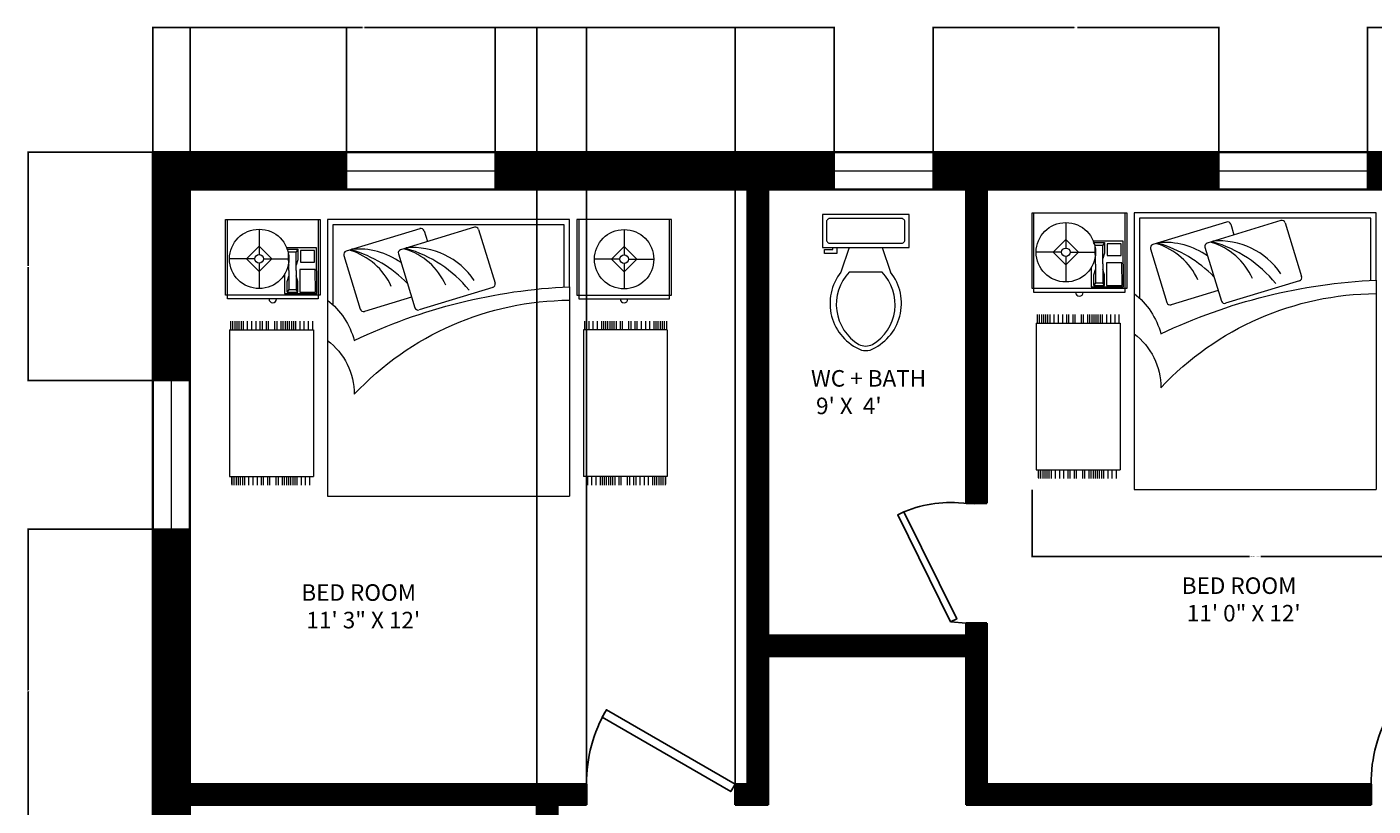
# Model space of a CAD drawing. Units: inches. Extents: x -24 to 516, y -23 to 640.
# Tile 4 of 5: x -24 to 302, y 452 to 640. Entities that reach past the tile are written whole.
import ezdxf

# ---------------------------------------------------------------- set-up
doc = ezdxf.new("R2010")
doc.units = ezdxf.units.IN
doc.header["$MEASUREMENT"] = 0
for name, color, linetype, lineweight in [('A-ANNO-DIMS', 2, 'Continuous', 18), ('A-AREA-IDEN', 7, 'Continuous', 18), ('A-WALL', 7, 'Continuous', 35), ('bathroom', 90, 'Continuous', 18), ('bedroom', 120, 'Continuous', 18), ('doors', 40, 'Continuous', 25), ('window', 30, 'Continuous', 18)]:
    doc.layers.add(name, color=color, linetype=linetype, lineweight=lineweight)
doc.layers.add('A-WALL-PATT', color=198, linetype='Continuous', lineweight=13, true_color=0x2e0f2e)
doc.styles.get("Standard").update_dxf_attribs({"font": 'arial.ttf'})
doc.dimstyles.get("Standard").update_dxf_attribs({"dimtxt": 0.18, "dimasz": 0.18, "dimexe": 0.18, "dimexo": 0.0625, "dimgap": 0.09, "dimtad": 0, "dimtih": 1, "dimtoh": 1, "dimdec": 4, "dimzin": 0, "dimdsep": 46, "dimtxsty": 'Standard', "dimcen": 0.09, "dimadec": 0, "dimazin": 0, "dimtfac": 1, "dimtdec": 4, "dimtofl": 0, "dimtmove": 0, "dimatfit": 3, "dimfxl": 1, "dimtolj": 1, "dimtzin": 0, "dimarcsym": 0})
pattern_1 = [(45, (-12045.43418, -42625.98622), (-0.08838834765, 0.08838834765), [])]

# ---------------------------------------------------------------- blocks, each defined once
blk = doc.blocks.new('*U7')
for p, q in [((0, 0), (0, 100)), ((750, 0), (750, 100))]:
    blk.add_line(p, q)
blk.add_lwpolyline([(0, 0), (649.5, -375), (671.4, -337.1), (21.9, 37.9)], close=True)
blk.add_arc((0, 0), 750, 330, 0)
blk = doc.blocks.new('*U6')
for p, q in [((0, 0), (0, -100)), ((750, 0), (750, -100))]:
    blk.add_line(p, q)
blk.add_lwpolyline([(0, 0), (649.5, 375), (671.4, 337.1), (21.9, -37.9)], close=True)
blk.add_arc((0, 0), 750, 0, 30)
blk = doc.blocks.new('3')
for p, q in [((185.8665, 224.6766), (185.8665, 225.2363)), ((185.8665, 225.2363), (186.566, 225.2363)), ((185.8805, 224.6487), (185.8805, 225.2363)), ((186.552, 225.2363), (186.552, 224.6487)), ((186.566, 225.2363), (186.566, 224.6766)), ((186.6199, 225.2363), (186.6199, 224.6399)), ((188.4089, 225.2363), (186.6199, 225.2363)), ((188.4089, 224.7393), (188.4089, 225.2363)), ((188.4627, 225.2363), (188.4627, 224.6766)), ((189.1623, 225.2363), (188.4627, 225.2363)), ((188.4767, 225.2363), (188.4767, 224.6486)), ((189.1483, 224.6486), (189.1483, 225.2363)), ((189.1623, 224.6766), (189.1623, 225.2363)), ((186.1157, 225.1643), (186.1157, 224.9763)), ((187.3034, 225.1683), (186.7581, 225.0015)), ((187.7059, 225.1793), (187.1607, 225.0124)), ((187.3344, 225.1518), (187.3586, 225.073)), ((187.737, 225.1628), (187.8585, 224.7657)), ((188.8125, 225.1618), (188.8125, 224.9738)), ((186.0216, 224.9449), (186.1157, 225.0389)), ((186.1157, 225.0389), (186.2097, 224.9449)), ((188.8125, 225.0365), (188.7185, 224.9424)), ((188.9065, 224.9424), (188.8125, 225.0365)), ((186.0843, 224.9449), (185.8963, 224.9449)), ((186.1157, 224.8509), (186.0216, 224.9449)), ((186.2097, 224.9449), (186.1157, 224.8509)), ((186.147, 224.9449), (186.335, 224.9449)), ((186.5397, 225.0274), (186.3193, 225.0266)), ((186.3215, 225.0167), (186.4008, 225.017)), ((186.3334, 224.9969), (186.3215, 225.0167)), ((186.3334, 224.9969), (186.389, 224.9971)), ((186.334, 224.858), (186.3334, 224.9969)), ((186.4008, 225.017), (186.389, 224.9971)), ((186.3895, 224.8582), (186.389, 224.9971)), ((186.4011, 224.9376), (186.3894, 224.8979)), ((186.4008, 225.017), (186.4011, 224.9376)), ((186.5409, 224.6901), (186.5397, 225.0274)), ((186.7416, 224.9704), (186.8631, 224.5734)), ((187.1442, 224.9814), (187.2657, 224.5843)), ((188.7812, 224.9424), (188.5931, 224.9424)), ((188.7185, 224.9424), (188.8125, 224.8484)), ((188.8125, 224.8484), (188.9065, 224.9424)), ((188.8438, 224.9424), (189.0319, 224.9424)), ((186.1157, 224.9136), (186.1157, 224.7256)), ((186.3023, 224.8297), (186.3029, 224.6892)), ((186.3314, 224.9055), (186.3338, 224.8977)), ((186.334, 224.858), (186.3345, 224.7191)), ((186.3895, 224.8582), (186.39, 224.7193)), ((188.8125, 224.9111), (188.8125, 224.723)), ((186.3224, 224.7786), (186.3341, 224.8183)), ((186.3227, 224.6992), (186.3224, 224.7786)), ((186.4017, 224.7789), (186.3897, 224.8185)), ((186.402, 224.6995), (186.4017, 224.7789)), ((187.842, 224.7347), (187.2967, 224.5678)), ((188.4089, 224.7393), (188.4089, 223.1907)), ((186.566, 224.6766), (185.8665, 224.6766)), ((186.552, 224.6487), (185.8805, 224.6487)), ((186.3029, 224.6892), (186.5409, 224.6901)), ((186.3345, 224.7191), (186.3227, 224.6992)), ((186.3227, 224.6992), (186.402, 224.6995)), ((186.3345, 224.7191), (186.39, 224.7193)), ((186.402, 224.6995), (186.39, 224.7193)), ((186.6199, 224.6399), (186.6199, 223.1907)), ((187.2416, 224.6632), (186.8942, 224.5569)), ((188.4627, 224.6766), (189.1623, 224.6766)), ((188.4767, 224.6486), (189.1483, 224.6486)), ((185.904, 224.4849, -0.9094), (185.904, 224.4204, -0.9094)), ((185.9195, 224.4849, -0.9094), (185.9195, 224.4204, -0.9094)), ((185.9195, 224.4849, -0.9094), (185.9195, 224.4204, -0.9094)), ((185.935, 224.4849, -0.9094), (185.935, 224.4204, -0.9094)), ((185.9505, 224.4849, -0.9094), (185.9505, 224.4204, -0.9094)), ((185.966, 224.4849, -0.9094), (185.966, 224.4204, -0.9094)), ((185.9815, 224.4849, -0.9094), (185.9815, 224.4204, -0.9094)), ((185.997, 224.4849, -0.9094), (185.997, 224.4204, -0.9094)), ((186.028, 224.4849, -0.9094), (186.028, 224.4204, -0.9094)), ((186.059, 224.4849, -0.9094), (186.059, 224.4204, -0.9094)), ((186.09, 224.4849, -0.9094), (186.09, 224.4204, -0.9094)), ((186.09, 224.4849, -0.9094), (186.09, 224.4204, -0.9094)), ((186.121, 224.4849, -0.9094), (186.121, 224.4204, -0.9094)), ((186.1365, 224.4849, -0.9094), (186.1365, 224.4204, -0.9094)), ((186.1675, 224.4849, -0.9094), (186.1675, 224.4204, -0.9094)), ((186.183, 224.4849, -0.9094), (186.183, 224.4204, -0.9094)), ((186.2295, 224.4849, -0.9094), (186.2295, 224.4204, -0.9094)), ((186.245, 224.4849, -0.9094), (186.245, 224.4204, -0.9094)), ((186.276, 224.4849, -0.9094), (186.276, 224.4204, -0.9094)), ((186.2915, 224.4849, -0.9094), (186.2915, 224.4204, -0.9094)), ((186.307, 224.4849, -0.9094), (186.307, 224.4204, -0.9094)), ((186.3225, 224.4849, -0.9094), (186.3225, 224.4204, -0.9094)), ((186.338, 224.4849, -0.9094), (186.338, 224.4204, -0.9094)), ((186.3535, 224.4849, -0.9094), (186.3535, 224.4204, -0.9094)), ((186.369, 224.4849, -0.9094), (186.369, 224.4204, -0.9094)), ((186.3845, 224.4849, -0.9094), (186.3845, 224.4204, -0.9094)), ((186.4155, 224.4849, -0.9094), (186.4155, 224.4204, -0.9094)), ((186.4465, 224.4849, -0.9094), (186.4465, 224.4204, -0.9094)), ((186.4775, 224.4849, -0.9094), (186.4775, 224.4204, -0.9094)), ((186.5085, 224.4849, -0.9094), (186.5085, 224.4204, -0.9094)), ((188.5202, 224.4849, -0.9094), (188.5202, 224.4204, -0.9094)), ((188.5512, 224.4849, -0.9094), (188.5512, 224.4204, -0.9094)), ((188.5822, 224.4849, -0.9094), (188.5822, 224.4204, -0.9094)), ((188.6132, 224.4849, -0.9094), (188.6132, 224.4204, -0.9094)), ((188.6442, 224.4849, -0.9094), (188.6442, 224.4204, -0.9094)), ((188.6597, 224.4849, -0.9094), (188.6597, 224.4204, -0.9094)), ((188.6752, 224.4849, -0.9094), (188.6752, 224.4204, -0.9094)), ((188.6907, 224.4849, -0.9094), (188.6907, 224.4204, -0.9094)), ((188.7062, 224.4849, -0.9094), (188.7062, 224.4204, -0.9094)), ((188.7217, 224.4849, -0.9094), (188.7217, 224.4204, -0.9094)), ((188.7372, 224.4849, -0.9094), (188.7372, 224.4204, -0.9094)), ((188.7527, 224.4849, -0.9094), (188.7527, 224.4204, -0.9094)), ((188.7837, 224.4849, -0.9094), (188.7837, 224.4204, -0.9094)), ((188.7992, 224.4849, -0.9094), (188.7992, 224.4204, -0.9094)), ((188.8457, 224.4849, -0.9094), (188.8457, 224.4204, -0.9094)), ((188.8612, 224.4849, -0.9094), (188.8612, 224.4204, -0.9094)), ((188.8922, 224.4849, -0.9094), (188.8922, 224.4204, -0.9094)), ((188.9077, 224.4849, -0.9094), (188.9077, 224.4204, -0.9094)), ((188.9387, 224.4849, -0.9094), (188.9387, 224.4204, -0.9094)), ((188.9387, 224.4849, -0.9094), (188.9387, 224.4204, -0.9094)), ((188.9697, 224.4849, -0.9094), (188.9697, 224.4204, -0.9094)), ((189.0007, 224.4849, -0.9094), (189.0007, 224.4204, -0.9094)), ((189.0317, 224.4849, -0.9094), (189.0317, 224.4204, -0.9094)), ((189.0472, 224.4849, -0.9094), (189.0472, 224.4204, -0.9094)), ((189.0627, 224.4849, -0.9094), (189.0627, 224.4204, -0.9094)), ((189.0782, 224.4849, -0.9094), (189.0782, 224.4204, -0.9094)), ((189.0937, 224.4849, -0.9094), (189.0937, 224.4204, -0.9094)), ((189.1092, 224.4849, -0.9094), (189.1092, 224.4204, -0.9094)), ((189.1092, 224.4849, -0.9094), (189.1092, 224.4204, -0.9094)), ((189.1247, 224.4849, -0.9094), (189.1247, 224.4204, -0.9094)), ((185.8974, 224.4204, -0.9094), (185.8974, 223.3378, -0.9094)), ((185.8974, 224.4204, -0.9094), (186.5174, 224.4204, -0.9094)), ((186.5174, 224.4204, -0.9094), (186.5174, 223.3378, -0.9094)), ((189.1313, 224.4204, -0.9094), (188.5113, 224.4204, -0.9094)), ((188.5113, 224.4204, -0.9094), (188.5113, 223.3378, -0.9094)), ((189.1313, 224.4204, -0.9094), (189.1313, 223.3378, -0.9094)), ((185.8974, 223.3378, -0.9094), (186.5174, 223.3378, -0.9094)), ((185.9114, 223.3378, -0.9094), (185.9114, 223.2789, -0.9094)), ((185.9114, 223.3378, -0.9094), (185.9114, 223.2789, -0.9094)), ((185.9114, 223.3378, -0.9094), (185.9114, 223.2789, -0.9094)), ((185.9138, 223.3378, -0.9094), (185.9138, 223.2732, -0.9094)), ((185.9293, 223.3378, -0.9094), (185.9293, 223.2732, -0.9094)), ((185.9293, 223.3378, -0.9094), (185.9293, 223.2732, -0.9094)), ((185.9448, 223.3378, -0.9094), (185.9448, 223.2732, -0.9094)), ((185.9603, 223.3378, -0.9094), (185.9603, 223.2732, -0.9094)), ((185.9758, 223.3378, -0.9094), (185.9758, 223.2732, -0.9094)), ((185.9913, 223.3378, -0.9094), (185.9913, 223.2732, -0.9094)), ((186.0068, 223.3378, -0.9094), (186.0068, 223.2732, -0.9094)), ((186.0378, 223.3378, -0.9094), (186.0378, 223.2732, -0.9094)), ((186.0688, 223.3378, -0.9094), (186.0688, 223.2732, -0.9094)), ((186.0998, 223.3378, -0.9094), (186.0998, 223.2732, -0.9094)), ((186.0998, 223.3378, -0.9094), (186.0998, 223.2732, -0.9094)), ((186.1308, 223.3378, -0.9094), (186.1308, 223.2732, -0.9094)), ((186.1463, 223.3378, -0.9094), (186.1463, 223.2732, -0.9094)), ((186.1773, 223.3378, -0.9094), (186.1773, 223.2732, -0.9094)), ((186.1928, 223.3378, -0.9094), (186.1928, 223.2732, -0.9094)), ((186.2393, 223.3378, -0.9094), (186.2393, 223.2732, -0.9094)), ((186.2548, 223.3378, -0.9094), (186.2548, 223.2732, -0.9094)), ((186.2858, 223.3378, -0.9094), (186.2858, 223.2732, -0.9094)), ((186.3013, 223.3378, -0.9094), (186.3013, 223.2732, -0.9094)), ((186.3168, 223.3378, -0.9094), (186.3168, 223.2732, -0.9094)), ((186.3323, 223.3378, -0.9094), (186.3323, 223.2732, -0.9094)), ((186.3478, 223.3378, -0.9094), (186.3478, 223.2732, -0.9094)), ((186.3633, 223.3378, -0.9094), (186.3633, 223.2732, -0.9094)), ((186.3788, 223.3378, -0.9094), (186.3788, 223.2732, -0.9094)), ((186.3943, 223.3378, -0.9094), (186.3943, 223.2732, -0.9094)), ((186.4253, 223.3378, -0.9094), (186.4253, 223.2732, -0.9094)), ((186.4563, 223.3378, -0.9094), (186.4563, 223.2732, -0.9094)), ((186.4873, 223.3378, -0.9094), (186.4873, 223.2732, -0.9094)), ((189.1313, 223.3378, -0.9094), (188.5113, 223.3378, -0.9094)), ((188.5414, 223.3378, -0.9094), (188.5414, 223.2732, -0.9094)), ((188.5724, 223.3378, -0.9094), (188.5724, 223.2732, -0.9094)), ((188.6034, 223.3378, -0.9094), (188.6034, 223.2732, -0.9094)), ((188.6344, 223.3378, -0.9094), (188.6344, 223.2732, -0.9094)), ((188.6499, 223.3378, -0.9094), (188.6499, 223.2732, -0.9094)), ((188.6654, 223.3378, -0.9094), (188.6654, 223.2732, -0.9094)), ((188.6809, 223.3378, -0.9094), (188.6809, 223.2732, -0.9094)), ((188.6964, 223.3378, -0.9094), (188.6964, 223.2732, -0.9094)), ((188.7119, 223.3378, -0.9094), (188.7119, 223.2732, -0.9094)), ((188.7274, 223.3378, -0.9094), (188.7274, 223.2732, -0.9094)), ((188.7429, 223.3378, -0.9094), (188.7429, 223.2732, -0.9094)), ((188.7739, 223.3378, -0.9094), (188.7739, 223.2732, -0.9094)), ((188.7894, 223.3378, -0.9094), (188.7894, 223.2732, -0.9094)), ((188.8359, 223.3378, -0.9094), (188.8359, 223.2732, -0.9094)), ((188.8514, 223.3378, -0.9094), (188.8514, 223.2732, -0.9094)), ((188.8824, 223.3378, -0.9094), (188.8824, 223.2732, -0.9094)), ((188.8979, 223.3378, -0.9094), (188.8979, 223.2732, -0.9094)), ((188.9289, 223.3378, -0.9094), (188.9289, 223.2732, -0.9094)), ((188.9289, 223.3378, -0.9094), (188.9289, 223.2732, -0.9094)), ((188.9599, 223.3378, -0.9094), (188.9599, 223.2732, -0.9094)), ((188.9909, 223.3378, -0.9094), (188.9909, 223.2732, -0.9094)), ((189.022, 223.3378, -0.9094), (189.022, 223.2732, -0.9094)), ((189.0375, 223.3378, -0.9094), (189.0375, 223.2732, -0.9094)), ((189.053, 223.3378, -0.9094), (189.053, 223.2732, -0.9094)), ((189.0685, 223.3378, -0.9094), (189.0685, 223.2732, -0.9094)), ((189.084, 223.3378, -0.9094), (189.084, 223.2732, -0.9094)), ((189.0995, 223.3378, -0.9094), (189.0995, 223.2732, -0.9094)), ((189.0995, 223.3378, -0.9094), (189.0995, 223.2732, -0.9094)), ((189.115, 223.3378, -0.9094), (189.115, 223.2732, -0.9094)), ((189.1173, 223.3378, -0.9094), (189.1173, 223.2789, -0.9094)), ((189.1173, 223.3378, -0.9094), (189.1173, 223.2789, -0.9094)), ((189.1173, 223.3378, -0.9094), (189.1173, 223.2789, -0.9094)), ((186.6199, 223.1907), (188.4089, 223.1907))]:
    blk.add_line(p, q)
blk.add_lwpolyline([(188.3691, 224.7374), (188.3691, 225.1965), (186.6596, 225.1965), (186.6596, 224.606)])
for points in [[(186.4217, 225.0072), (186.422, 224.9199), (186.5252, 224.9202), (186.5249, 225.0075)], [(186.4153, 224.8663), (186.4159, 224.6996), (186.531, 224.7), (186.5304, 224.8667)]]:
    blk.add_lwpolyline(points, close=True)
for points in [[(186.6199, 224.6399, -0.162278), (186.8186, 224.3418, -0.100664), (188.4089, 224.7393, -0.100664)], [(186.6199, 224.3418, -0.236068), (186.8186, 223.9442, -0.205258), (188.4089, 224.6399, -0.205258)]]:
    blk.add_lwpolyline(points, format="xyb")
for centre, radius in [((186.1157, 224.9449), 0.2194), ((188.8125, 224.9424), 0.2194), ((186.1157, 224.9449), 0.0313), ((188.8125, 224.9424), 0.0313)]:
    blk.add_circle(centre, radius)
for centre, radius, start, end in [((187.3107, 225.1446), 0.0248, 17.0142, 107.0142), ((187.7132, 225.1555), 0.0248, 17.0142, 107.0142), ((187.2502, 224.4821), 0.5468, 33.78007, 95.16051), ((186.7654, 224.9777), 0.0248, 107.0142, 197.0142), ((186.6474, 224.5408), 0.4873, 24.22087, 73.06906), ((186.8477, 224.4712), 0.5468, 54.68511, 95.16051), ((186.5359, 224.1054), 0.9426, 44.27274, 73.71889), ((187.1679, 224.9887), 0.0248, 107.0142, 197.0142), ((187.0499, 224.5517), 0.4873, 24.22087, 73.06906), ((186.9385, 224.1164), 0.9426, 39.40233, 73.71889), ((187.8347, 224.7585), 0.0248, 287.0142, 17.0142), ((186.2163, 224.6487), 0.028, 180, 0), ((188.8125, 224.6486), 0.028, 180, 0), ((186.8869, 224.5806), 0.0248, 197.0142, 287.0142), ((187.2894, 224.5916), 0.0248, 197.0142, 287.0142)]:
    blk.add_arc(centre, radius, start, end)
blk = doc.blocks.new('Toilet - top')
for p, q in [((9.5, -6), (9.5, -2)), ((-10, -8.5), (-8, -8.5)), ((-10, -9.5), (-10, -8.5)), ((-7, -9.5), (-10, -9.5)), ((-8, -8.5), (-8, -8)), ((-7, -8), (-7, -9.5)), ((-4, -8), (-6, -14)), ((4, -8), (6, -14)), ((4, -14), (-4, -14))]:
    blk.add_line(p, q)
blk.add_lwpolyline([(10.5, -8), (10.5, 0), (-10.5, 0), (-10.5, -8)], close=True)
for points in [[(-9.5, -2), (-9.5, -6)], [(8.5, -1), (-8.5, -1)], [(-8.5, -7), (8.5, -7)]]:
    blk.add_lwpolyline(points)
for centre, radius, start, end in [((-8.62, -1.88), 0.884, 81.8699, 188.1301), ((8.62, -1.88), 0.884, 351.8699, 98.1301), ((-8.62, -6.12), 0.884, 171.8699, 278.1301), ((8.62, -6.12), 0.884, 261.8699, 8.1301), ((3.52, -21.58), 12.17, 141.4691, 247.9714), ((4.2, -21.82), 11.33, 136.3677, 238.9468), ((-3.52, -21.58), 12.17, 292.0284, 38.5307), ((-4.2, -21.82), 11.33, 301.053, 43.6321), ((0, -27.88), 4, 245.7318, 294.2682), ((0, -29), 4, 254.8605, 285.1395)]:
    blk.add_arc(centre, radius, start, end)
blk = doc.blocks.new('WIN-36IN')
for p, q in [((0, 0), (0, 36)), ((0, 36), (9, 36)), ((4.5, 0), (4.5, 36)), ((9, 36), (9, 0)), ((9, 0), (0, 0)), ((9, 0), (4.5, 0))]:
    blk.add_line(p, q)
blk = doc.blocks.new('WIN-24IN')
for p, q in [((0, 0), (0, 24)), ((0, 24), (9, 24)), ((4.5, 0), (4.5, 24)), ((9, 24), (9, 0)), ((9, 0), (0, 0)), ((9, 0), (4.5, 0))]:
    blk.add_line(p, q)
blk = doc.blocks.new('*D15')
at = {"layer": 'A-ANNO-DIMS', "color": 0, "lineweight": -2, "transparency": 16777216}
for p, q in [((219.01, 528.26), (219.01, 511.94)), ((327.01, 528.26), (327.01, 511.94)), ((219.19, 512.12), (271.63, 512.12)), ((326.83, 512.12), (274.4, 512.12))]:
    blk.add_line(p, q, dxfattribs=at)
at = {"layer": 'A-ANNO-DIMS', "color": 0, "transparency": 16777216}
for points in [[(219.19, 512.15), (219.19, 512.09), (219.01, 512.12)], [(326.83, 512.15), (326.83, 512.09), (327.01, 512.12)]]:
    blk.add_solid(points, dxfattribs=at)
at = {"layer": 'Defpoints', "color": 0, "transparency": 16777216}
for p in [(219.01, 528.32), (327.01, 528.32), (327.01, 512.12)]:
    blk.add_point(p, dxfattribs=at)
at = {"layer": 'A-ANNO-DIMS', "color": 0, "transparency": 16777216, "insert": (273.01, 512.12), "char_height": 0.18, "attachment_point": 5}
blk.add_mtext('\\A1;BED GROUP 108 TYP.', dxfattribs=at)
blk = doc.blocks.new('*D44')
at = {"layer": 'A-ANNO-DIMS', "color": 0, "lineweight": -2, "transparency": 16777216}
for p, q in [((6.03, 518.75), (-24.28, 518.75)), ((-24.1, 518.57), (-24.1, 479.8)), ((-24.1, 440.65), (-24.1, 479.43)), ((6.03, 440.47), (-24.28, 440.47))]:
    blk.add_line(p, q, dxfattribs=at)
at = {"layer": 'A-ANNO-DIMS', "color": 0, "transparency": 16777216}
for points in [[(-24.13, 518.57), (-24.07, 518.57), (-24.1, 518.75)], [(-24.13, 440.65), (-24.07, 440.65), (-24.1, 440.47)]]:
    blk.add_solid(points, dxfattribs=at)
at = {"layer": 'Defpoints', "color": 0, "transparency": 16777216}
for p in [(-24.1, 518.75), (6.09, 518.75), (6.09, 440.47)]:
    blk.add_point(p, dxfattribs=at)
at = {"layer": 'A-ANNO-DIMS', "color": 0, "transparency": 16777216, "insert": (-24.1, 479.61), "char_height": 0.18, "attachment_point": 5}
blk.add_mtext('\\A1;78.28', dxfattribs=at)
blk = doc.blocks.new('*D45')
at = {"layer": 'A-ANNO-DIMS', "color": 0, "lineweight": -2, "transparency": 16777216}
for p, q in [((6.03, 610.01), (-24.28, 610.01)), ((-24.1, 609.83), (-24.1, 582.56)), ((-24.1, 554.93), (-24.1, 582.2)), ((6.03, 554.75), (-24.28, 554.75))]:
    blk.add_line(p, q, dxfattribs=at)
at = {"layer": 'A-ANNO-DIMS', "color": 0, "transparency": 16777216}
for points in [[(-24.13, 609.83), (-24.07, 609.83), (-24.1, 610.01)], [(-24.13, 554.93), (-24.07, 554.93), (-24.1, 554.75)]]:
    blk.add_solid(points, dxfattribs=at)
at = {"layer": 'Defpoints', "color": 0, "transparency": 16777216}
for p in [(-24.1, 610.01), (6.09, 610.01), (6.09, 554.75)]:
    blk.add_point(p, dxfattribs=at)
at = {"layer": 'A-ANNO-DIMS', "color": 0, "transparency": 16777216, "insert": (-24.1, 582.38), "char_height": 0.18, "attachment_point": 5}
blk.add_mtext('\\A1;55.26', dxfattribs=at)
blk = doc.blocks.new('*D46')
at = {"layer": 'A-ANNO-DIMS', "color": 0, "lineweight": -2, "transparency": 16777216}
for p, q in [((15.09, 398.08), (15.09, 640.38)), ((15.27, 640.2), (56.87, 640.2)), ((98.91, 640.2), (57.31, 640.2)), ((99.09, 398.08), (99.09, 640.38))]:
    blk.add_line(p, q, dxfattribs=at)
at = {"layer": 'A-ANNO-DIMS', "color": 0, "transparency": 16777216}
for points in [[(15.27, 640.23), (15.27, 640.17), (15.09, 640.2)], [(98.91, 640.23), (98.91, 640.17), (99.09, 640.2)]]:
    blk.add_solid(points, dxfattribs=at)
at = {"layer": 'Defpoints', "color": 0, "transparency": 16777216}
for p in [(99.09, 640.2), (15.09, 398.01), (99.09, 398.01)]:
    blk.add_point(p, dxfattribs=at)
at = {"layer": 'A-ANNO-DIMS', "color": 0, "transparency": 16777216, "insert": (57.09, 640.2), "char_height": 0.18, "attachment_point": 5}
blk.add_mtext('\\A1;84', dxfattribs=at)
blk = doc.blocks.new('*D57')
at = {"layer": 'A-ANNO-DIMS', "color": 0, "lineweight": -2, "transparency": 16777216}
for p, q in [((111.09, 452.08), (111.09, 640.38)), ((111.27, 640.2), (128.87, 640.2)), ((146.91, 640.2), (129.31, 640.2)), ((147.09, 452.08), (147.09, 640.38))]:
    blk.add_line(p, q, dxfattribs=at)
at = {"layer": 'A-ANNO-DIMS', "color": 0, "transparency": 16777216}
for points in [[(111.27, 640.23), (111.27, 640.17), (111.09, 640.2)], [(146.91, 640.23), (146.91, 640.17), (147.09, 640.2)]]:
    blk.add_solid(points, dxfattribs=at)
at = {"layer": 'Defpoints', "color": 0, "transparency": 16777216}
for p in [(147.09, 640.2), (111.09, 452.01), (147.09, 452.01)]:
    blk.add_point(p, dxfattribs=at)
at = {"layer": 'A-ANNO-DIMS', "color": 0, "transparency": 16777216, "insert": (129.09, 640.2), "char_height": 0.18, "attachment_point": 5}
blk.add_mtext('\\A1;36', dxfattribs=at)
blk = doc.blocks.new('*D61')
at = {"layer": 'A-ANNO-DIMS', "color": 0, "lineweight": -2, "transparency": 16777216}
for p, q in [((6.09, 610.08), (6.09, 640.38)), ((6.27, 640.2), (29.16, 640.2)), ((52.82, 640.2), (29.92, 640.2)), ((53, 610.08), (53, 640.38))]:
    blk.add_line(p, q, dxfattribs=at)
at = {"layer": 'A-ANNO-DIMS', "color": 0, "transparency": 16777216}
for points in [[(6.27, 640.23), (6.27, 640.17), (6.09, 640.2)], [(52.82, 640.23), (52.82, 640.17), (53, 640.2)]]:
    blk.add_solid(points, dxfattribs=at)
at = {"layer": 'Defpoints', "color": 0, "transparency": 16777216}
for p in [(53, 640.2), (6.09, 610.01), (53, 610.01)]:
    blk.add_point(p, dxfattribs=at)
at = {"layer": 'A-ANNO-DIMS', "color": 0, "transparency": 16777216, "insert": (29.54, 640.2), "char_height": 0.18, "attachment_point": 5}
blk.add_mtext('\\A1;46.91', dxfattribs=at)
blk = doc.blocks.new('*D62')
at = {"layer": 'A-ANNO-DIMS', "color": 0, "lineweight": -2, "transparency": 16777216}
for p, q in [((89, 610.08), (89, 640.38)), ((89.18, 640.2), (129.64, 640.2)), ((170.88, 640.2), (130.43, 640.2)), ((171.06, 610.08), (171.06, 640.38))]:
    blk.add_line(p, q, dxfattribs=at)
at = {"layer": 'A-ANNO-DIMS', "color": 0, "transparency": 16777216}
for points in [[(89.18, 640.23), (89.18, 640.17), (89, 640.2)], [(170.88, 640.23), (170.88, 640.17), (171.06, 640.2)]]:
    blk.add_solid(points, dxfattribs=at)
at = {"layer": 'Defpoints', "color": 0, "transparency": 16777216}
for p in [(171.06, 640.2), (89, 610.01), (171.06, 610.01)]:
    blk.add_point(p, dxfattribs=at)
at = {"layer": 'A-ANNO-DIMS', "color": 0, "transparency": 16777216, "insert": (130.03, 640.2), "char_height": 0.18, "attachment_point": 5}
blk.add_mtext('\\A1;82.07', dxfattribs=at)
blk = doc.blocks.new('*D63')
at = {"layer": 'A-ANNO-DIMS', "color": 0, "lineweight": -2, "transparency": 16777216}
for p, q in [((195.06, 610.08), (195.06, 640.38)), ((195.24, 640.2), (229.24, 640.2)), ((264.03, 640.2), (230.03, 640.2)), ((264.21, 610.08), (264.21, 640.38))]:
    blk.add_line(p, q, dxfattribs=at)
at = {"layer": 'A-ANNO-DIMS', "color": 0, "transparency": 16777216}
for points in [[(195.24, 640.23), (195.24, 640.17), (195.06, 640.2)], [(264.03, 640.23), (264.03, 640.17), (264.21, 640.2)]]:
    blk.add_solid(points, dxfattribs=at)
at = {"layer": 'Defpoints', "color": 0, "transparency": 16777216}
for p in [(264.21, 640.2), (195.06, 610.01), (264.21, 610.01)]:
    blk.add_point(p, dxfattribs=at)
at = {"layer": 'A-ANNO-DIMS', "color": 0, "transparency": 16777216, "insert": (229.64, 640.2), "char_height": 0.18, "attachment_point": 5}
blk.add_mtext('\\A1;69.14', dxfattribs=at)
blk = doc.blocks.new('*D64')
at = {"layer": 'A-ANNO-DIMS', "color": 0, "lineweight": -2, "transparency": 16777216}
for p, q in [((300.21, 610.08), (300.21, 640.38)), ((300.39, 640.2), (341.99, 640.2)), ((384.38, 640.2), (342.78, 640.2)), ((384.56, 610.08), (384.56, 640.38))]:
    blk.add_line(p, q, dxfattribs=at)
at = {"layer": 'A-ANNO-DIMS', "color": 0, "transparency": 16777216}
for points in [[(300.39, 640.23), (300.39, 640.17), (300.21, 640.2)], [(384.38, 640.23), (384.38, 640.17), (384.56, 640.2)]]:
    blk.add_solid(points, dxfattribs=at)
at = {"layer": 'Defpoints', "color": 0, "transparency": 16777216}
for p in [(384.56, 640.2), (300.21, 610.01), (384.56, 610.01)]:
    blk.add_point(p, dxfattribs=at)
at = {"layer": 'A-ANNO-DIMS', "color": 0, "transparency": 16777216, "insert": (342.38, 640.2), "char_height": 0.18, "attachment_point": 5}
blk.add_mtext('\\A1;84.35', dxfattribs=at)

msp = doc.modelspace()

# ---------------------------------------------------------------- hatches: boundary and pattern name
at = {"layer": 'A-WALL-PATT'}
h = msp.add_hatch(dxfattribs=at)
h.set_pattern_fill('ANSI31', color=256)
h.set_pattern_definition(pattern_1)
h.paths.add_polyline_path([(15.088, 601.013), (52.998, 601.013), (52.998, 610.013), (6.088, 610.013), (6.088, 554.753), (15.088, 554.753)])
h.paths.add_polyline_path([(171.065, 610.013), (88.998, 610.013), (88.998, 601.013), (150.088, 601.013), (150.088, 457.013), (147.088, 457.013), (147.088, 452.013), (155.088, 452.013), (155.088, 488.013), (203.088, 488.013), (203.088, 452.013), (301.088, 452.013), (301.088, 457.013), (208.088, 457.013), (208.088, 496.013), (203.088, 496.013), (203.088, 493.013), (155.088, 493.013), (155.088, 601.013), (171.065, 601.013)])
h.paths.add_polyline_path([(264.208, 610.013), (195.065, 610.013), (195.065, 601.013), (203.088, 601.013), (203.088, 525.013), (208.088, 525.013), (208.088, 601.013), (264.208, 601.013)], flags=17)
h.paths.add_polyline_path([(384.556, 610.013), (300.208, 610.013), (300.208, 601.013), (340.088, 601.013), (340.088, 457.013), (337.088, 456.991), (337.088, 452.013), (340.088, 452.013), (348.088, 452.013), (348.088, 457.013), (345.088, 457.013), (345.088, 601.013), (384.556, 601.013)])
h.paths.add_polyline_path([(486.088, 610.013), (420.556, 610.013), (420.556, 601.013), (477.088, 601.013), (477.088, 564.302), (486.088, 564.302)])
h.paths.add_polyline_path([(486.088, 516.302), (477.088, 516.302), (477.088, 457.013), (387.088, 457.013), (387.088, 430.013), (392.088, 430.013), (392.088, 452.013), (477.088, 452.013), (477.088, 442.706), (486.088, 442.706)])
h.paths.add_polyline_path([(486.088, 418.706), (477.088, 418.706), (477.088, 398.013), (392.088, 398.013), (392.088, 401.013), (388.222, 401.013), (387.088, 401.013), (387.088, 398.013), (336.088, 398.013), (336.088, 386.013), (345.088, 386.013), (345.088, 389.013), (477.088, 389.013), (477.088, 320.013), (486.088, 320.013)])
h.paths.add_polyline_path([(486.088, 272.013), (477.088, 272.013), (477.088, 182.013), (398.088, 182.013), (398.088, 173.013), (486.088, 173.013)])
h = msp.add_hatch(dxfattribs=at)
h.set_pattern_fill('ANSI31', color=256)
h.set_pattern_definition(pattern_1)
h.paths.add_polyline_path([(161.63, 139.013), (155.088, 139.013), (155.088, 283.013), (203.088, 283.013), (203.088, 171.013), (208.088, 171.013), (208.088, 283.013), (211.088, 283.013), (211.088, 288.013), (208.088, 288.013), (147.088, 288.013), (147.088, 283.013), (150.088, 283.013), (150.088, 139.013), (87.664, 139.013), (87.664, 134.513), (87.664, 130.013), (161.63, 130.013)])
h.paths.add_polyline_path([(256.352, 139.013), (208.088, 139.013), (208.088, 142.013), (203.088, 142.013), (203.088, 139.013), (185.63, 139.013), (185.63, 130.013), (256.352, 130.013)])
h.paths.add_polyline_path([(345.088, 326.013), (336.088, 326.013), (336.088, 288.013), (247.088, 288.013), (247.088, 283.013), (340.088, 283.013), (340.088, 139.013), (292.352, 139.013), (292.352, 134.513), (292.352, 130.013), (345.088, 130.013)])
h.paths.add_polyline_path([(51.664, 139.013), (15.088, 139.013), (15.088, 195.946), (10.588, 195.946), (6.088, 195.946), (6.088, 130.013), (51.664, 130.013)])
h.paths.add_polyline_path([(15.088, 283.013), (111.088, 283.013), (111.088, 288.013), (104.088, 288.013), (104.088, 354.013), (99.088, 354.013), (99.088, 288.013), (15.088, 288.013), (15.088, 324.046), (10.588, 324.046), (6.088, 324.046), (6.088, 231.946), (15.088, 231.946)])
h.paths.add_polyline_path([(15.088, 398.013), (99.088, 398.013), (99.088, 390.013), (104.088, 390.013), (104.088, 393.013), (104.088, 407.013), (99.088, 407.013), (99.088, 404.013), (15.088, 404.013), (15.088, 416.474), (10.588, 416.474), (6.088, 416.474), (6.088, 360.046), (15.088, 360.046)])
h.paths.add_polyline_path([(15.088, 518.753), (10.588, 518.753), (6.088, 518.753), (6.088, 440.474), (15.088, 440.474), (15.088, 452.013), (99.088, 452.013), (99.088, 436.013), (104.088, 436.013), (104.088, 452.013), (111.088, 452.013), (111.088, 457.013), (15.088, 457.013)])

# ---------------------------------------------------------------- linework, layer by layer
at = {"layer": 'A-WALL'}
for p, q in [((15.088, 601.013), (150.088, 601.013)), ((15.088, 457.013), (15.088, 601.013)), ((150.088, 457.013), (150.088, 601.013)), ((155.088, 601.013), (203.088, 601.013)), ((155.088, 493.013), (155.088, 601.013)), ((203.088, 525.013), (203.088, 601.013)), ((208.088, 601.013), (340.088, 601.013)), ((208.088, 525.013), (208.088, 601.013)), ((208.088, 525.013), (203.088, 525.013)), ((203.088, 493.013), (203.088, 496.013)), ((203.088, 493.013), (203.088, 496.013)), ((203.088, 496.013), (208.088, 496.013)), ((208.088, 457.013), (208.088, 496.013)), ((155.088, 493.013), (203.088, 493.013)), ((155.088, 488.013), (203.088, 488.013)), ((155.088, 452.013), (155.088, 488.013)), ((203.088, 452.013), (203.088, 488.013)), ((15.088, 457.013), (111.088, 457.013)), ((111.088, 452.013), (111.088, 457.013)), ((147.088, 457.013), (150.088, 457.013)), ((150.088, 457.013), (147.088, 457.013)), ((147.088, 457.013), (147.088, 452.013)), ((208.088, 457.013), (301.088, 457.013)), ((301.088, 457.013), (301.088, 452.013)), ((15.088, 452.013), (99.088, 452.013)), ((15.088, 404.013), (15.088, 452.013)), ((99.088, 436.013), (99.088, 452.013)), ((104.088, 452.013), (111.088, 452.013)), ((104.088, 436.013), (104.088, 452.013)), ((147.088, 452.013), (155.088, 452.013)), ((203.088, 452.013), (301.088, 452.013))]:
    msp.add_line(p, q, dxfattribs=at)
msp.add_lwpolyline([(345.088, 130.013), (6.088, 130.013), (6.088, 610.013), (486.088, 610.013), (486.088, 173.013)], dxfattribs=at)

# ---------------------------------------------------------------- block references
at = {"layer": 'bathroom'}
msp.add_blockref('Toilet - top', (178.722, 594.987), dxfattribs=at)
at = {"layer": 'bedroom', "xscale": 32.76894482774335, "yscale": 32.76894482774335, "zscale": 32.76894482774335}
for p in [(-6066.971, -6787.006), (-5871.636, -6785.399)]:
    msp.add_blockref('3', p, dxfattribs=at)
at = {"layer": 'doors'}
for name, p, xscale, yscale, zscale, rotation in [('*U6', (199.239, 496.27), 0.0385810261037899, 0.0385810261037899, 0.0385810261037899, 86.1859251657114), ('*U7', (147.088, 457.013), 0.0480000000000013, 0.0480000000000013, 0.0480000000000013, 180), ('*U7', (337.088, 456.991), 0.0480000093397263, 0.0480000093397263, 0.0480000093397263, 179.9642575698038)]:
    msp.add_blockref(name, p, dxfattribs=dict(at, xscale=xscale, yscale=yscale, zscale=zscale, rotation=rotation))
at = {"layer": 'window', "extrusion": (0, 0, -1), "zscale": -1}
for name, p, rotation in [('WIN-36IN', (-52.998, 601.013), 89.99999999998766), ('WIN-24IN', (-171.065, 601.013), 90.00000000000529), ('WIN-36IN', (-264.208, 601.013), 89.9999999999877)]:
    msp.add_blockref(name, p, dxfattribs=dict(at, rotation=rotation))
at = {"layer": 'window'}
msp.add_blockref('WIN-36IN', (6.088, 518.753), dxfattribs=at)

# ---------------------------------------------------------------- texts
at = {"layer": 'A-AREA-IDEN', "char_height": 4, "attachment_point": 1}
for s, insert in [("  WC + BATH\\P   9' X  4'", (163.023, 557.27)), (' BED ROOM\\P  11\' 3" X 12\'', (40.836, 505.399)), (' BED ROOM\\P  11\' 0" X 12\'', (254.038, 507.069))]:
    msp.add_mtext_dynamic_manual_height_columns(s, width=74.82673, gutter_width=1, heights=[0], dxfattribs=dict(at, insert=insert))

# ---------------------------------------------------------------- dimensions: what is measured, and where the dimension line sits
at = {"layer": 'A-ANNO-DIMS'}
for base, p1, p2, override, picture, middle in [((52.998, 640.198), (6.088, 610.013), (52.998, 610.013), {"dimdec": 2, "dimlfac": 1, "dimrnd": 0, "dimzin": 0, "dimdsep": 46, "dimlunit": 2}, '*D61', (29.543, 640.198)), ((99.088, 640.198), (15.088, 398.013), (99.088, 398.013), {"dimdec": 0, "dimlfac": 1, "dimrnd": 0, "dimzin": 0, "dimdsep": 46, "dimlunit": 2}, '*D46', (57.088, 640.198)), ((171.065, 640.198), (88.998, 610.013), (171.065, 610.013), {"dimdec": 2, "dimlfac": 1, "dimrnd": 0, "dimzin": 0, "dimdsep": 46, "dimlunit": 2}, '*D62', (130.031, 640.198)), ((147.088, 640.198), (111.088, 452.013), (147.088, 452.013), {"dimdec": 0, "dimlfac": 1, "dimrnd": 0, "dimzin": 0, "dimdsep": 46, "dimlunit": 2}, '*D57', (129.088, 640.198)), ((264.208, 640.198), (195.065, 610.013), (264.208, 610.013), {"dimdec": 2, "dimlfac": 1, "dimrnd": 0, "dimzin": 0, "dimdsep": 46, "dimlunit": 2}, '*D63', (229.636, 640.198)), ((384.556, 640.198), (300.208, 610.013), (384.556, 610.013), {"dimdec": 2, "dimlfac": 1, "dimrnd": 0, "dimzin": 0, "dimdsep": 46, "dimlunit": 2}, '*D64', (342.382, 640.198))]:
    dim = msp.add_linear_dim(base=base, p1=p1, p2=p2, dimstyle='Standard', override=override, dxfattribs=at)
    dim.commit()
    dim.dimension.update_dxf_attribs({"geometry": picture, "text_midpoint": middle})
for base, p1, p2, picture, middle in [((-24.097, 610.013), (6.088, 554.753), (6.088, 610.013), '*D45', (-24.097, 582.383)), ((-24.097, 518.753), (6.088, 440.474), (6.088, 518.753), '*D44', (-24.097, 479.614))]:
    dim = msp.add_linear_dim(base=base, p1=p1, p2=p2, angle=90, dimstyle='Standard', override={"dimdec": 2, "dimlfac": 1, "dimrnd": 0, "dimzin": 0, "dimdsep": 46, "dimlunit": 2}, dxfattribs=at)
    dim.commit()
    dim.dimension.update_dxf_attribs({"geometry": picture, "text_midpoint": middle})
dim = msp.add_linear_dim(base=(327.013, 512.124), p1=(219.013, 528.324), p2=(327.013, 528.324), text='BED GROUP <> TYP.', dimstyle='Standard', override={"dimdec": 0, "dimlfac": 1, "dimrnd": 0, "dimzin": 0, "dimdsep": 46, "dimlunit": 2}, dxfattribs=at)
dim.commit()
dim.dimension.update_dxf_attribs({"geometry": '*D15', "text_midpoint": (273.013, 512.124)})

doc.saveas('drawing.dxf')
